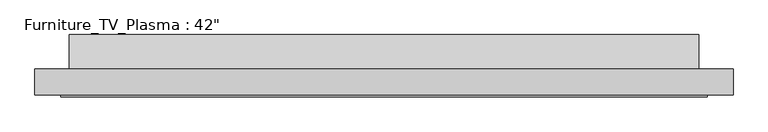
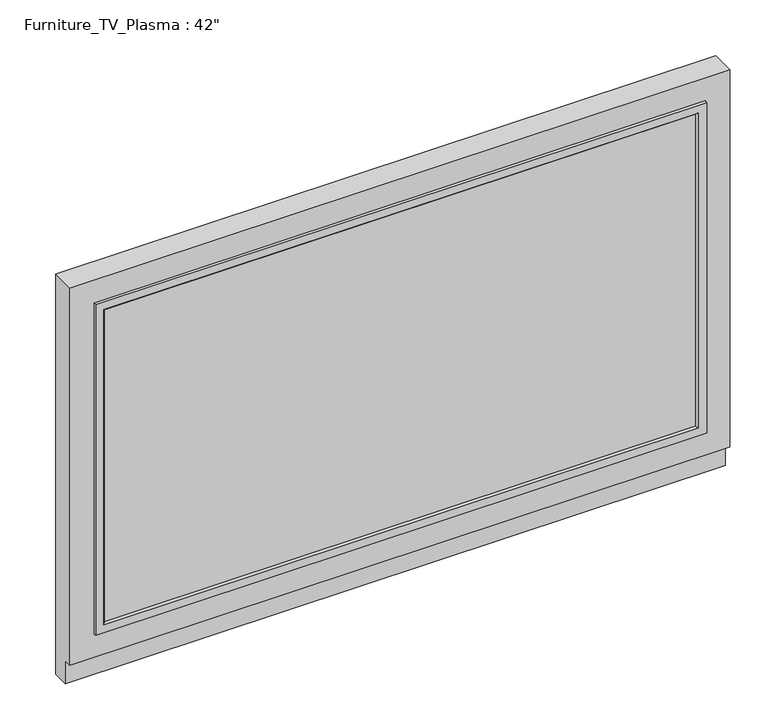
"""IFC4 building model written with IfcOpenShell, lengths in millimetres: furniture geometry."""

from ifc_helpers import new_model, si_unit, frame, origin, place, context, project, spatial, polyline, outline, extrude, faceted_brep, source, transform, mapped, element, save


def furniture_0b97a49d(model_context):
    return source(origin(), model_context, "Body", "SolidModel", [
        faceted_brep([(571.5, -50.8, 660.4), (-457.2, -50.8, 660.4), (-457.2, -88.9, 660.4), (571.5, -88.9, 660.4), (-457.2, -50.8, 0.0), (571.5, -50.8, 0.0), (571.5, -76.2, 0.0), (-457.2, -76.2, 0.0), (-457.2, -76.2, 38.1), (-457.2, -88.9, 38.1), (571.5, -88.9, 38.1), (533.4, -88.9, 622.3), (533.4, -88.9, 76.2), (-419.1, -88.9, 76.2), (-419.1, -88.9, 622.3), (571.5, -76.2, 38.1), (533.4, -74.1720413, 622.3), (-419.1, -74.1720413, 622.3), (-419.1, -74.1720413, 76.2), (533.4, -74.1720413, 76.2)], [[[0, 1, 2, 3]], [[4, 5, 6, 7]], [[1, 0, 5, 4]], [[2, 1, 4, 7, 8, 9]], [[3, 2, 9, 10], [11, 12, 13, 14]], [[0, 3, 10, 15, 6, 5]], [[16, 17, 18, 19]], [[16, 19, 12, 11]], [[19, 18, 13, 12]], [[18, 17, 14, 13]], [[17, 16, 11, 14]], [[15, 8, 7, 6]], [[8, 15, 10, 9]]]),
        extrude(outline(polyline([(520.7, -88.9), (-406.4, -88.9), (-406.4, -74.1720413), (520.7, -74.1720413), (520.7, -88.9)])), frame((0.0, 0.0, 88.9), z_axis=(0.0, 0.0, 1.0), x_axis=(1.0, 0.0, 0.0)), (0.0, 0.0, 1.0), 520.7),
        extrude(outline(polyline([(0.0, 574.8688953), (0.0, 38.1), (-50.8, 38.1), (-50.8, 609.6), (0.0, 574.8688953)])), frame((-406.4, 0.0, 0.0), z_axis=(1.0, 0.0, 0.0), x_axis=(0.0, 1.0, 0.0)), (0.0, 0.0, 1.0), 927.1),
        faceted_brep([(517.525, -88.9, 92.075), (520.7, -92.075, 88.9), (520.7, -92.075, 608.80625), (517.525, -88.9, 605.63125), (520.7, -74.1720413, 88.9), (520.7, -88.9, 88.9), (520.7, -88.9, 608.80625), (520.7, -74.1720413, 608.80625), (533.4, -92.075, 76.2), (533.4, -74.1720413, 76.2), (533.4, -74.1720413, 621.50625), (533.4, -92.075, 621.50625), (-406.4, -92.075, 608.80625), (-403.225, -88.9, 605.63125), (-406.4, -88.9, 608.80625), (-406.4, -74.1720413, 608.80625), (-419.1, -74.1720413, 621.50625), (-419.1, -92.075, 621.50625), (-406.4, -92.075, 88.9), (-403.225, -88.9, 92.075), (-406.4, -88.9, 88.9), (-406.4, -74.1720413, 88.9), (-419.1, -74.1720413, 76.2), (-419.1, -92.075, 76.2)], [[[0, 1, 2, 3]], [[4, 5, 6, 7]], [[8, 9, 10, 11]], [[3, 2, 12, 13]], [[7, 6, 14, 15]], [[11, 10, 16, 17]], [[13, 12, 18, 19]], [[15, 14, 20, 21]], [[17, 16, 22, 23]], [[11, 17, 23, 8], [1, 18, 12, 2]], [[19, 18, 1, 0]], [[5, 20, 14, 6], [3, 13, 19, 0]], [[21, 20, 5, 4]], [[9, 22, 16, 10], [7, 15, 21, 4]], [[23, 22, 9, 8]]]),
    ])


if __name__ == "__main__":
    model = new_model("IFC4")
    model_context = context("Model", 3, world=origin())
    ifc_project = project(units=[si_unit("LENGTHUNIT", "METRE", prefix="MILLI")], contexts=[model_context])
    site = spatial("IfcSite", under=ifc_project)
    building = spatial("IfcBuilding", under=site)
    placement = place(None, origin())
    furniture_shape = furniture_0b97a49d(model_context)
    element("IfcFurniture", 1, ObjectType="Furniture_TV_Plasma : 42\"", at=placement, inside=building, context=model_context, shape_type="MappedRepresentation", body=[
        mapped(furniture_shape, transform((0.0, 0.0, 0.0), x_axis=(1.0, 0.0, 0.0), y_axis=(0.0, 1.0, 0.0), z_axis=(0.0, 0.0, 1.0))),
    ])
    save(model, "model.ifc")

# Revit data of these elements
# Type "Furniture_TV_Plasma : 42\""
#   Keynote = "N"
#   Assembly Code = "E2020200"
#   Depth = 0.291667 ft
#   Height = 2.166667 ft
#   Width = 3.375 ft
#   Material Cabinet = Plastic - Gray
#   Default Elevation = 0
# Element 1 (IfcFurniture, "Furniture_TV_Plasma : 42\"")
#   Materials on its faces: "Plastic - Black", "Plastic - Gray", "Glass"
# Materials
#   "Plastic - Gray": class "Plastic", colour RGB 134 134 134, transparency 0
#   "Plastic - Black": colour RGB 0 0 0, transparency 0
#   "Glass": class "Glass", colour RGB 0 128 192, transparency 0.9, Description = "Soda Lime Glass", Cost = 0
